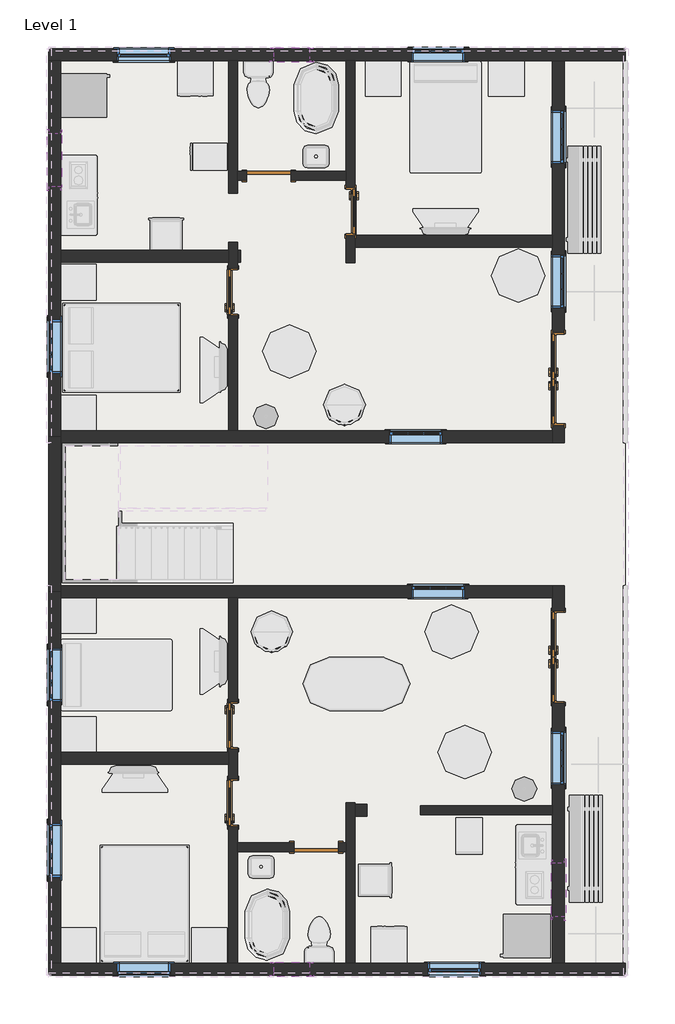
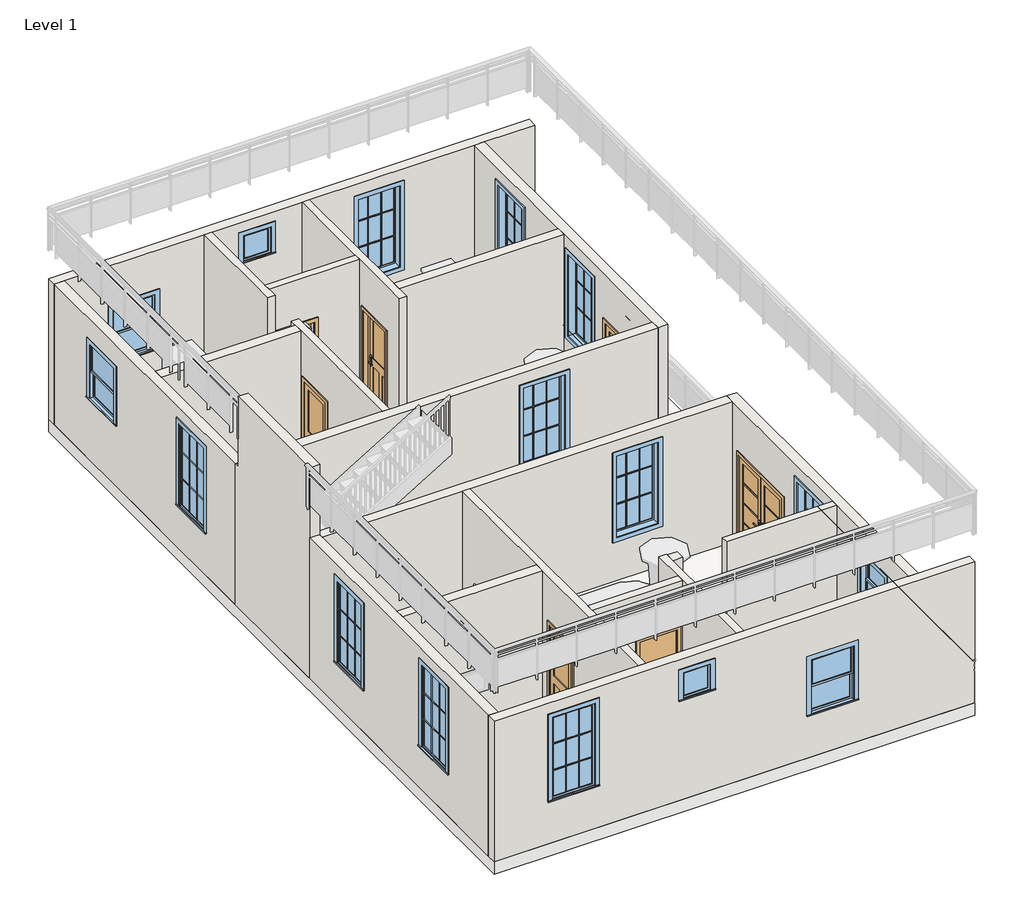
# One storey, part 1 of 4: 22 walls, 16 windows, 8 doors, 1 slab.
"""IFC4 building model written with IfcOpenShell, lengths in millimetres."""

from ifc_helpers import new_model, si_unit, frame, origin, origin_with_axes, place, context, project, spatial, polyline, outline, extrude, faceted_brep, transform, mapped, element, save
from components import door_ce1fc124, door_cdf9d6cc, door_b03bd389, door_255cab33, window_8b323df3, window_31198920, window_e41d21a6

model = new_model("IFC4")

# Units and contexts
model_context = context("Model", 3, world=origin())
ifc_project = project(units=[si_unit("LENGTHUNIT", "METRE", prefix="MILLI")], contexts=[model_context])

# Site, building, storey
site = spatial("IfcSite", under=ifc_project)
building = spatial("IfcBuilding", under=site)
storey = spatial("IfcBuildingStorey", under=building, Name="Level 1", Elevation=0.0)

# Doors
placement = place(None, origin())
door_shape = door_ce1fc124(model_context)
element("IfcDoor", 1, ObjectType="30\" x 80\"", at=placement, inside=storey, context=model_context, shape_type="MappedRepresentation", body=[
    mapped(door_shape, transform((-11423.8500862, 2290.6620171, 0.0), x_axis=(0.0, -1.0, 0.0), y_axis=(1.0, 0.0, 0.0), z_axis=(0.0, 0.0, 1.0))),
])
element("IfcDoor", 2, ObjectType="30\" x 80\"", at=placement, inside=storey, context=model_context, shape_type="MappedRepresentation", body=[
    mapped(door_shape, transform((-11423.8500862, 11015.5620171, 0.0), x_axis=(0.0, -1.0, 0.0), y_axis=(1.0, 0.0, 0.0), z_axis=(0.0, 0.0, 1.0))),
])
element("IfcDoor", 3, ObjectType="30\" x 80\"", at=placement, inside=storey, context=model_context, shape_type="MappedRepresentation", body=[
    mapped(door_shape, transform((-9410.9000862, 12387.1620171, 0.0), x_axis=(0.0, 1.0, 0.0), y_axis=(-1.0, 0.0, 0.0), z_axis=(0.0, 0.0, 1.0))),
])
door_2_shape = door_cdf9d6cc(model_context)
element("IfcDoor", 4, ObjectType="30\" x 80\"", at=placement, inside=storey, context=model_context, shape_type="MappedRepresentation", body=[
    mapped(door_2_shape, transform((-11423.8500862, 3611.4620171, 0.0), x_axis=(0.0, 1.0, 0.0), y_axis=(-1.0, 0.0, 0.0), z_axis=(0.0, 0.0, 1.0))),
])
door_3_shape = door_b03bd389(model_context)
element("IfcDoor", 5, ObjectType="Door-Exterior-Double-Full Glass-Wood_Clad : 60\" x 80\"", at=placement, inside=storey, context=model_context, shape_type="MappedRepresentation", body=[
    mapped(door_3_shape, transform((-5861.2500862, 9529.6620171, 0.0), x_axis=(0.0, 1.0, 0.0), y_axis=(-1.0, 0.0, 0.0), z_axis=(0.0, 0.0, 1.0))),
])
element("IfcDoor", 6, ObjectType="Door-Exterior-Double-Full Glass-Wood_Clad : 60\" x 80\"", at=placement, inside=storey, context=model_context, shape_type="MappedRepresentation", body=[
    mapped(door_3_shape, transform((-5861.2500862, 4779.8620171, 0.0), x_axis=(0.0, 1.0, 0.0), y_axis=(-1.0, 0.0, 0.0), z_axis=(0.0, 0.0, 1.0))),
])
door_4_shape = door_255cab33(model_context)
element("IfcDoor", 7, ObjectType="Single-Flush : 30\" x 80\"", at=placement, inside=storey, context=model_context, shape_type="MappedRepresentation", body=[
    mapped(door_4_shape, transform((-10811.0750862, 12996.7620171, 0.0), x_axis=(-1.0, 0.0, 0.0), y_axis=(0.0, -1.0, 0.0), z_axis=(0.0, 0.0, 1.0))),
])
element("IfcDoor", 8, ObjectType="Single-Flush : 30\" x 80\"", at=placement, inside=storey, context=model_context, shape_type="MappedRepresentation", body=[
    mapped(door_4_shape, transform((-9998.2750862, 1528.6620171, 0.0), x_axis=(1.0, 0.0, 0.0), y_axis=(0.0, 1.0, 0.0), z_axis=(0.0, 0.0, 1.0))),
])

# Slab
element("IfcSlab", 9, ObjectType="Wood Joist 10\" - Ceramic Tile", at=placement, inside=storey, context=model_context, shape_type="SweptSolid", body=[
    extrude(outline(polyline([(-4715.0750862, 15168.4620171), (-4715.0750862, -655.7379829), (-14570.2750862, -655.7379829), (-14570.2750862, 15168.4620171), (-4715.0750862, 15168.4620171)])), frame((0.0, 0.0, -273.05), z_axis=(0.0, 0.0, 1.0), x_axis=(1.0, 0.0, 0.0)), (0.0, 0.0, 1.0), 273.05),
])

# Walls
element("IfcWall", 10, ObjectType="Generic - 8\"", at=placement, inside=storey, context=model_context, shape_type="Brep", body=[
    faceted_brep([(-14570.2750862, 14965.2620171, 0.0), (-14367.0750862, 14965.2620171, 0.0), (-11496.8750862, 14965.2620171, 0.0), (-11344.4750862, 14965.2620171, 0.0), (-9490.2750862, 14965.2620171, 0.0), (-9337.8750862, 14965.2620171, 0.0), (-5959.6750862, 14965.2620171, 0.0), (-5756.4750862, 14965.2620171, 0.0), (-4715.0750862, 14965.2620171, 0.0), (-4715.0750862, 14965.2620171, 3048.0), (-5756.4750862, 14965.2620171, 3048.0), (-5959.6750862, 14965.2620171, 3048.0), (-9337.8750862, 14965.2620171, 3048.0), (-9490.2750862, 14965.2620171, 3048.0), (-11344.4750862, 14965.2620171, 3048.0), (-11496.8750862, 14965.2620171, 3048.0), (-14367.0750862, 14965.2620171, 3048.0), (-14570.2750862, 14965.2620171, 3048.0), (-7458.2750862, 14965.2620171, 2743.2), (-7458.2750862, 14965.2620171, 914.4), (-8372.6750862, 14965.2620171, 914.4), (-8372.6750862, 14965.2620171, 2743.2), (-13401.8750862, 14965.2620171, 2133.6), (-12487.4750862, 14965.2620171, 2133.6), (-12487.4750862, 14965.2620171, 914.4), (-13401.8750862, 14965.2620171, 914.4), (-10722.1750862, 14965.2620171, 2768.6), (-10112.5750862, 14965.2620171, 2768.6), (-10112.5750862, 14965.2620171, 2159.0), (-10722.1750862, 14965.2620171, 2159.0), (-14570.2750862, 15168.4620171, 0.0), (-14570.2750862, 15168.4620171, 3048.0), (-4715.0750862, 15168.4620171, 3048.0), (-4715.0750862, 15168.4620171, 0.0), (-7458.2750862, 15168.4620171, 2743.2), (-8372.6750862, 15168.4620171, 2743.2), (-8372.6750862, 15168.4620171, 914.4), (-7458.2750862, 15168.4620171, 914.4), (-13401.8750862, 15168.4620171, 2133.6), (-13401.8750862, 15168.4620171, 914.4), (-12487.4750862, 15168.4620171, 914.4), (-12487.4750862, 15168.4620171, 2133.6), (-10722.1750862, 15168.4620171, 2768.6), (-10722.1750862, 15168.4620171, 2159.0), (-10112.5750862, 15168.4620171, 2159.0), (-10112.5750862, 15168.4620171, 2768.6)], [[[0, 1, 2, 3, 4, 5, 6, 7, 8, 9, 10, 11, 12, 13, 14, 15, 16, 17], [18, 19, 20, 21], [22, 23, 24, 25], [26, 27, 28, 29]], [[30, 31, 32, 33], [34, 35, 36, 37], [38, 39, 40, 41], [42, 43, 44, 45]], [[8, 7, 6, 5, 4, 3, 2, 1, 0, 30, 33]], [[9, 8, 33, 32]], [[0, 17, 31, 30]], [[19, 18, 34, 37]], [[20, 19, 37, 36]], [[21, 20, 36, 35]], [[18, 21, 35, 34]], [[39, 38, 22, 25]], [[40, 39, 25, 24]], [[41, 40, 24, 23]], [[38, 41, 23, 22]], [[43, 42, 26, 29]], [[44, 43, 29, 28]], [[45, 44, 28, 27]], [[42, 45, 27, 26]], [[17, 16, 15, 14, 13, 12, 11, 10, 9, 32, 31]]]),
])
element("IfcWall", 11, ObjectType="Generic - 8\"", at=placement, inside=storey, context=model_context, shape_type="Brep", body=[
    faceted_brep([(-4715.0750862, -452.5379829, 0.0), (-5756.4750862, -452.5379829, 0.0), (-5959.6750862, -452.5379829, 0.0), (-9337.8750862, -452.5379829, 0.0), (-9490.2750862, -452.5379829, 0.0), (-11344.4750862, -452.5379829, 0.0), (-11496.8750862, -452.5379829, 0.0), (-14367.0750862, -452.5379829, 0.0), (-14570.2750862, -452.5379829, 0.0), (-14570.2750862, -452.5379829, 3048.0), (-14367.0750862, -452.5379829, 3048.0), (-11496.8750862, -452.5379829, 3048.0), (-11344.4750862, -452.5379829, 3048.0), (-9490.2750862, -452.5379829, 3048.0), (-9337.8750862, -452.5379829, 3048.0), (-5959.6750862, -452.5379829, 3048.0), (-5756.4750862, -452.5379829, 3048.0), (-4715.0750862, -452.5379829, 3048.0), (-13401.8750862, -452.5379829, 2743.2), (-13401.8750862, -452.5379829, 914.4), (-12487.4750862, -452.5379829, 914.4), (-12487.4750862, -452.5379829, 2743.2), (-8093.2750862, -452.5379829, 2133.6), (-8093.2750862, -452.5379829, 914.4), (-7178.8750862, -452.5379829, 914.4), (-7178.8750862, -452.5379829, 2133.6), (-10722.1750862, -452.5379829, 2768.6), (-10722.1750862, -452.5379829, 2159.0), (-10112.5750862, -452.5379829, 2159.0), (-10112.5750862, -452.5379829, 2768.6), (-4715.0750862, -655.7379829, 0.0), (-4715.0750862, -655.7379829, 3048.0), (-14570.2750862, -655.7379829, 3048.0), (-14570.2750862, -655.7379829, 0.0), (-13401.8750862, -655.7379829, 2743.2), (-12487.4750862, -655.7379829, 2743.2), (-12487.4750862, -655.7379829, 914.4), (-13401.8750862, -655.7379829, 914.4), (-8093.2750862, -655.7379829, 2133.6), (-7178.8750862, -655.7379829, 2133.6), (-7178.8750862, -655.7379829, 914.4), (-8093.2750862, -655.7379829, 914.4), (-10722.1750862, -655.7379829, 2768.6), (-10112.5750862, -655.7379829, 2768.6), (-10112.5750862, -655.7379829, 2159.0), (-10722.1750862, -655.7379829, 2159.0)], [[[0, 1, 2, 3, 4, 5, 6, 7, 8, 9, 10, 11, 12, 13, 14, 15, 16, 17], [18, 19, 20, 21], [22, 23, 24, 25], [26, 27, 28, 29]], [[30, 31, 32, 33], [34, 35, 36, 37], [38, 39, 40, 41], [42, 43, 44, 45]], [[8, 7, 6, 5, 4, 3, 2, 1, 0, 30, 33]], [[0, 17, 31, 30]], [[9, 8, 33, 32]], [[17, 16, 15, 14, 13, 12, 11, 10, 9, 32, 31]], [[19, 18, 34, 37]], [[20, 19, 37, 36]], [[21, 20, 36, 35]], [[18, 21, 35, 34]], [[23, 22, 38, 41]], [[24, 23, 41, 40]], [[25, 24, 40, 39]], [[22, 25, 39, 38]], [[27, 26, 42, 45]], [[28, 27, 45, 44]], [[29, 28, 44, 43]], [[26, 29, 43, 42]]]),
])
element("IfcWall", 12, ObjectType="Generic - 8\"", at=placement, inside=storey, context=model_context, shape_type="Brep", body=[
    faceted_brep([(-14367.0750862, -452.5379829, 0.0), (-14367.0750862, 2951.0620171, 0.0), (-14367.0750862, 3154.2620171, 0.0), (-14367.0750862, 5795.8620171, 0.0), (-14367.0750862, 5897.4620171, 0.0), (-14367.0750862, 5897.4620171, 3048.0), (-14367.0750862, 5795.8620171, 3048.0), (-14367.0750862, 3154.2620171, 3048.0), (-14367.0750862, 2951.0620171, 3048.0), (-14367.0750862, -452.5379829, 3048.0), (-14367.0750862, 1935.0620171, 2743.2), (-14367.0750862, 1935.0620171, 914.4), (-14367.0750862, 1020.6620171, 914.4), (-14367.0750862, 1020.6620171, 2743.2), (-14367.0750862, 4932.2620171, 2743.2), (-14367.0750862, 4932.2620171, 914.4), (-14367.0750862, 4017.8620171, 914.4), (-14367.0750862, 4017.8620171, 2743.2), (-14570.2750862, -452.5379829, 0.0), (-14570.2750862, -452.5379829, 3048.0), (-14570.2750862, 5897.4620171, 3048.0), (-14570.2750862, 5897.4620171, 0.0), (-14570.2750862, 1935.0620171, 2743.2), (-14570.2750862, 1020.6620171, 2743.2), (-14570.2750862, 1020.6620171, 914.4), (-14570.2750862, 1935.0620171, 914.4), (-14570.2750862, 4932.2620171, 2743.2), (-14570.2750862, 4017.8620171, 2743.2), (-14570.2750862, 4017.8620171, 914.4), (-14570.2750862, 4932.2620171, 914.4)], [[[0, 1, 2, 3, 4, 5, 6, 7, 8, 9], [10, 11, 12, 13], [14, 15, 16, 17]], [[18, 19, 20, 21], [22, 23, 24, 25], [26, 27, 28, 29]], [[4, 3, 2, 1, 0, 18, 21]], [[5, 4, 21, 20]], [[9, 8, 7, 6, 5, 20, 19]], [[0, 9, 19, 18]], [[11, 10, 22, 25]], [[12, 11, 25, 24]], [[13, 12, 24, 23]], [[10, 13, 23, 22]], [[15, 14, 26, 29]], [[16, 15, 29, 28]], [[17, 16, 28, 27]], [[14, 17, 27, 26]]]),
])
element("IfcWall", 13, ObjectType="Generic - 8\"", at=placement, inside=storey, context=model_context, shape_type="Brep", body=[
    faceted_brep([(-5959.6750862, 14965.2620171, 3048.0), (-5959.6750862, 14965.2620171, 0.0), (-5959.6750862, 11980.7620171, 0.0), (-5959.6750862, 11777.5620171, 0.0), (-5959.6750862, 10317.0620171, 0.0), (-5959.6750862, 10317.0620171, 2057.4), (-5959.6750862, 8742.2620171, 2057.4), (-5959.6750862, 8742.2620171, 0.0), (-5959.6750862, 8640.6620171, 0.0), (-5959.6750862, 8437.4620171, 0.0), (-5959.6750862, 8437.4620171, 3048.0), (-5959.6750862, 8640.6620171, 3048.0), (-5959.6750862, 11777.5620171, 3048.0), (-5959.6750862, 11980.7620171, 3048.0), (-5959.6750862, 10736.1620171, 2743.2), (-5959.6750862, 10736.1620171, 914.4), (-5959.6750862, 11650.5620171, 914.4), (-5959.6750862, 11650.5620171, 2743.2), (-5959.6750862, 13206.3120171, 2743.2), (-5959.6750862, 13206.3120171, 914.4), (-5959.6750862, 14120.7120171, 914.4), (-5959.6750862, 14120.7120171, 2743.2), (-5756.4750862, 14965.2620171, 0.0), (-5756.4750862, 14965.2620171, 3048.0), (-5756.4750862, 8437.4620171, 3048.0), (-5756.4750862, 8437.4620171, 0.0), (-5756.4750862, 8742.2620171, 0.0), (-5756.4750862, 8742.2620171, 2057.4), (-5756.4750862, 10317.0620171, 2057.4), (-5756.4750862, 10317.0620171, 0.0), (-5756.4750862, 10736.1620171, 2743.2), (-5756.4750862, 11650.5620171, 2743.2), (-5756.4750862, 11650.5620171, 914.4), (-5756.4750862, 10736.1620171, 914.4), (-5756.4750862, 13206.3120171, 2743.2), (-5756.4750862, 14120.7120171, 2743.2), (-5756.4750862, 14120.7120171, 914.4), (-5756.4750862, 13206.3120171, 914.4)], [[[0, 1, 2, 3, 4, 5, 6, 7, 8, 9, 10, 11, 12, 13], [14, 15, 16, 17], [18, 19, 20, 21]], [[22, 23, 24, 25, 26, 27, 28, 29], [30, 31, 32, 33], [34, 35, 36, 37]], [[1, 22, 29, 4, 3, 2]], [[25, 9, 8, 7, 26]], [[1, 0, 23, 22]], [[10, 9, 25, 24]], [[28, 5, 4, 29]], [[5, 28, 27, 6]], [[6, 27, 26, 7]], [[15, 14, 30, 33]], [[16, 15, 33, 32]], [[17, 16, 32, 31]], [[14, 17, 31, 30]], [[19, 18, 34, 37]], [[20, 19, 37, 36]], [[21, 20, 36, 35]], [[18, 21, 35, 34]], [[0, 13, 12, 11, 10, 24, 23]]]),
])
element("IfcWall", 14, ObjectType="Generic - 8\"", at=placement, inside=storey, context=model_context, shape_type="Brep", body=[
    faceted_brep([(-5959.6750862, 8640.6620171, 0.0), (-11344.4750862, 8640.6620171, 0.0), (-11496.8750862, 8640.6620171, 0.0), (-14367.0750862, 8640.6620171, 0.0), (-14367.0750862, 8640.6620171, 3048.0), (-11496.8750862, 8640.6620171, 3048.0), (-11344.4750862, 8640.6620171, 3048.0), (-5959.6750862, 8640.6620171, 3048.0), (-7839.2750862, 8640.6620171, 2743.2), (-8753.6750862, 8640.6620171, 2743.2), (-8753.6750862, 8640.6620171, 914.4), (-7839.2750862, 8640.6620171, 914.4), (-5959.6750862, 8437.4620171, 0.0), (-5959.6750862, 8437.4620171, 3048.0), (-14367.0750862, 8437.4620171, 3048.0), (-14367.0750862, 8437.4620171, 0.0), (-7839.2750862, 8437.4620171, 2743.2), (-7839.2750862, 8437.4620171, 914.4), (-8753.6750862, 8437.4620171, 914.4), (-8753.6750862, 8437.4620171, 2743.2), (-14367.0750862, 8539.0620171, 0.0), (-14367.0750862, 8539.0620171, 3048.0)], [[[0, 1, 2, 3, 4, 5, 6, 7], [8, 9, 10, 11]], [[12, 13, 14, 15], [16, 17, 18, 19]], [[3, 2, 1, 0, 12, 15, 20]], [[0, 7, 13, 12]], [[17, 16, 8, 11]], [[18, 17, 11, 10]], [[19, 18, 10, 9]], [[16, 19, 9, 8]], [[7, 6, 5, 4, 21, 14, 13]], [[4, 3, 20, 15, 14, 21]]]),
])
element("IfcWall", 15, ObjectType="Generic - 8\"", at=placement, inside=storey, context=model_context, shape_type="Brep", body=[
    faceted_brep([(-5959.6750862, 5999.0620171, 0.0), (-14367.0750862, 5999.0620171, 0.0), (-14367.0750862, 5999.0620171, 3048.0), (-5959.6750862, 5999.0620171, 3048.0), (-7458.2750862, 5999.0620171, 2743.2), (-8372.6750862, 5999.0620171, 2743.2), (-8372.6750862, 5999.0620171, 914.4), (-7458.2750862, 5999.0620171, 914.4), (-5959.6750862, 5795.8620171, 0.0), (-5959.6750862, 5795.8620171, 3048.0), (-11344.4750862, 5795.8620171, 3048.0), (-11496.8750862, 5795.8620171, 3048.0), (-14367.0750862, 5795.8620171, 3048.0), (-14367.0750862, 5795.8620171, 0.0), (-11496.8750862, 5795.8620171, 0.0), (-11344.4750862, 5795.8620171, 0.0), (-7458.2750862, 5795.8620171, 2743.2), (-7458.2750862, 5795.8620171, 914.4), (-8372.6750862, 5795.8620171, 914.4), (-8372.6750862, 5795.8620171, 2743.2), (-14367.0750862, 5897.4620171, 0.0), (-14367.0750862, 5897.4620171, 3048.0)], [[[0, 1, 2, 3], [4, 5, 6, 7]], [[8, 9, 10, 11, 12, 13, 14, 15], [16, 17, 18, 19]], [[1, 0, 8, 15, 14, 13, 20]], [[0, 3, 9, 8]], [[3, 2, 21, 12, 11, 10, 9]], [[17, 16, 4, 7]], [[18, 17, 7, 6]], [[19, 18, 6, 5]], [[16, 19, 5, 4]], [[2, 1, 20, 13, 12, 21]]]),
])
element("IfcWall", 16, ObjectType="Generic - 8\"", at=placement, inside=storey, context=model_context, shape_type="Brep", body=[
    faceted_brep([(-5959.6750862, -452.5379829, 0.0), (-5959.6750862, -452.5379829, 3048.0), (-5959.6750862, 2087.4620171, 3048.0), (-5959.6750862, 2239.8620171, 3048.0), (-5959.6750862, 5795.8620171, 3048.0), (-5959.6750862, 5999.0620171, 3048.0), (-5959.6750862, 5999.0620171, 0.0), (-5959.6750862, 5795.8620171, 0.0), (-5959.6750862, 5567.2620171, 0.0), (-5959.6750862, 5567.2620171, 2057.4), (-5959.6750862, 3992.4620171, 2057.4), (-5959.6750862, 3992.4620171, 0.0), (-5959.6750862, 2239.8620171, 0.0), (-5959.6750862, 2087.4620171, 0.0), (-5959.6750862, 2595.4620171, 2743.2), (-5959.6750862, 2595.4620171, 914.4), (-5959.6750862, 3509.8620171, 914.4), (-5959.6750862, 3509.8620171, 2743.2), (-5959.6750862, 347.5620171, 2540.0), (-5959.6750862, 347.5620171, 1320.8), (-5959.6750862, 1261.9620171, 1320.8), (-5959.6750862, 1261.9620171, 2540.0), (-5756.4750862, -452.5379829, 3048.0), (-5756.4750862, -452.5379829, 0.0), (-5756.4750862, 3992.4620171, 0.0), (-5756.4750862, 3992.4620171, 2057.4), (-5756.4750862, 5567.2620171, 2057.4), (-5756.4750862, 5567.2620171, 0.0), (-5756.4750862, 5999.0620171, 0.0), (-5756.4750862, 5999.0620171, 3048.0), (-5756.4750862, 2595.4620171, 2743.2), (-5756.4750862, 3509.8620171, 2743.2), (-5756.4750862, 3509.8620171, 914.4), (-5756.4750862, 2595.4620171, 914.4), (-5756.4750862, 347.5620171, 2540.0), (-5756.4750862, 1261.9620171, 2540.0), (-5756.4750862, 1261.9620171, 1320.8), (-5756.4750862, 347.5620171, 1320.8)], [[[0, 1, 2, 3, 4, 5, 6, 7, 8, 9, 10, 11, 12, 13], [14, 15, 16, 17], [18, 19, 20, 21]], [[22, 23, 24, 25, 26, 27, 28, 29], [30, 31, 32, 33], [34, 35, 36, 37]], [[23, 0, 13, 12, 11, 24]], [[6, 28, 27, 8, 7]], [[1, 0, 23, 22]], [[6, 5, 29, 28]], [[26, 9, 8, 27]], [[9, 26, 25, 10]], [[10, 25, 24, 11]], [[5, 4, 3, 2, 1, 22, 29]], [[15, 14, 30, 33]], [[16, 15, 33, 32]], [[17, 16, 32, 31]], [[14, 17, 31, 30]], [[19, 18, 34, 37]], [[20, 19, 37, 36]], [[21, 20, 36, 35]], [[18, 21, 35, 34]]]),
])
element("IfcWall", 17, ObjectType="Generic - 8\"", at=placement, inside=storey, context=model_context, shape_type="SweptSolid", body=[
    extrude(outline(polyline([(-14367.0750862, 3154.2620171), (-11496.8750862, 3154.2620171), (-11496.8750862, 2951.0620171), (-14367.0750862, 2951.0620171), (-14367.0750862, 3154.2620171)])), origin_with_axes(), (0.0, 0.0, 1.0), 3048.0),
])
element("IfcWall", 18, ObjectType="Generic - 8\"", at=placement, inside=storey, context=model_context, shape_type="SweptSolid", body=[
    extrude(outline(polyline([(-14367.0750862, 11726.7620171), (-11496.8750862, 11726.7620171), (-11496.8750862, 11523.5620171), (-14367.0750862, 11523.5620171), (-14367.0750862, 11726.7620171)])), origin_with_axes(), (0.0, 0.0, 1.0), 3048.0),
])
element("IfcWall", 19, ObjectType="Generic - 8\"", at=placement, inside=storey, context=model_context, shape_type="SweptSolid", body=[
    extrude(outline(polyline([(-11293.6750862, 11523.5620171), (-11344.4750862, 11523.5620171), (-11344.4750862, 11726.7620171), (-11293.6750862, 11726.7620171), (-11293.6750862, 11523.5620171)])), origin_with_axes(), (0.0, 0.0, 1.0), 3048.0),
])
element("IfcWall", 20, ObjectType="Generic - 8\"", at=placement, inside=storey, context=model_context, shape_type="Brep", body=[
    faceted_brep([(-9337.8750862, 11777.5620171, 0.0), (-5959.6750862, 11777.5620171, 0.0), (-5959.6750862, 11777.5620171, 3048.0), (-9337.8750862, 11777.5620171, 3048.0), (-9337.8750862, 11980.7620171, 0.0), (-9337.8750862, 11980.7620171, 2057.4), (-9337.8750862, 11980.7620171, 3048.0), (-5959.6750862, 11980.7620171, 3048.0), (-5959.6750862, 11980.7620171, 0.0)], [[[0, 1, 2, 3]], [[4, 5, 6, 7, 8]], [[1, 0, 4, 8]], [[2, 1, 8, 7]], [[0, 3, 6, 5, 4]], [[3, 2, 7, 6]]]),
])
element("IfcWall", 21, ObjectType="Generic - 8\"", at=placement, inside=storey, context=model_context, shape_type="SweptSolid", body=[
    extrude(outline(polyline([(-9337.8750862, 2265.2620171), (-9134.6750862, 2265.2620171), (-9134.6750862, 2062.0620171), (-9337.8750862, 2062.0620171), (-9337.8750862, 2265.2620171)])), origin_with_axes(), (0.0, 0.0, 1.0), 3048.0),
])
element("IfcWall", 22, ObjectType="Generic - 8\"", at=placement, inside=storey, context=model_context, shape_type="Brep", body=[
    faceted_brep([(-14367.0750862, 8539.0620171, 0.0), (-14367.0750862, 8640.6620171, 0.0), (-14367.0750862, 11523.5620171, 0.0), (-14367.0750862, 11726.7620171, 0.0), (-14367.0750862, 14965.2620171, 0.0), (-14367.0750862, 14965.2620171, 3048.0), (-14367.0750862, 11726.7620171, 3048.0), (-14367.0750862, 11523.5620171, 3048.0), (-14367.0750862, 8640.6620171, 3048.0), (-14367.0750862, 8539.0620171, 3048.0), (-14367.0750862, 10539.3120171, 2743.2), (-14367.0750862, 10539.3120171, 914.4), (-14367.0750862, 9624.9120171, 914.4), (-14367.0750862, 9624.9120171, 2743.2), (-14367.0750862, 13727.0120171, 2540.0), (-14367.0750862, 13727.0120171, 1320.8), (-14367.0750862, 12812.6120171, 1320.8), (-14367.0750862, 12812.6120171, 2540.0), (-14570.2750862, 8539.0620171, 0.0), (-14570.2750862, 8539.0620171, 3048.0), (-14570.2750862, 14965.2620171, 3048.0), (-14570.2750862, 14965.2620171, 0.0), (-14570.2750862, 10539.3120171, 2743.2), (-14570.2750862, 9624.9120171, 2743.2), (-14570.2750862, 9624.9120171, 914.4), (-14570.2750862, 10539.3120171, 914.4), (-14570.2750862, 13727.0120171, 2540.0), (-14570.2750862, 12812.6120171, 2540.0), (-14570.2750862, 12812.6120171, 1320.8), (-14570.2750862, 13727.0120171, 1320.8)], [[[0, 1, 2, 3, 4, 5, 6, 7, 8, 9], [10, 11, 12, 13], [14, 15, 16, 17]], [[18, 19, 20, 21], [22, 23, 24, 25], [26, 27, 28, 29]], [[4, 3, 2, 1, 0, 18, 21]], [[0, 9, 19, 18]], [[5, 4, 21, 20]], [[10, 13, 23, 22]], [[13, 12, 24, 23]], [[12, 11, 25, 24]], [[11, 10, 22, 25]], [[14, 17, 27, 26]], [[17, 16, 28, 27]], [[16, 15, 29, 28]], [[15, 14, 26, 29]], [[9, 8, 7, 6, 5, 20, 19]]]),
])
element("IfcWall", 23, ObjectType="Generic - 8\"", at=placement, inside=storey, context=model_context, shape_type="Brep", body=[
    faceted_brep([(-14367.0750862, 5897.4620171, 0.0), (-14367.0750862, 5999.0620171, 0.0), (-14367.0750862, 8437.4620171, 0.0), (-14367.0750862, 8539.0620171, 0.0), (-14367.0750862, 8539.0620171, 3048.0), (-14367.0750862, 8437.4620171, 3048.0), (-14367.0750862, 8437.4620171, 4572.0), (-14367.0750862, 5897.4620171, 4572.0), (-14367.0750862, 5897.4620171, 3048.0), (-14570.2750862, 5897.4620171, 0.0), (-14570.2750862, 5897.4620171, 3048.0), (-14570.2750862, 5897.4620171, 4572.0), (-14570.2750862, 8437.4620171, 4572.0), (-14570.2750862, 8437.4620171, 3048.0), (-14570.2750862, 8539.0620171, 3048.0), (-14570.2750862, 8539.0620171, 0.0)], [[[0, 1, 2, 3, 4, 5, 6, 7, 8]], [[9, 10, 11, 12, 13, 14, 15]], [[3, 2, 1, 0, 9, 15]], [[4, 3, 15, 14]], [[0, 8, 7, 11, 10, 9]], [[7, 6, 12, 11]], [[12, 6, 5, 13]], [[5, 4, 14, 13]]]),
])
element("IfcWall", 24, ObjectType="inner wall", at=placement, inside=storey, context=model_context, shape_type="Brep", body=[
    faceted_brep([(-11496.8750862, 14965.2620171, 0.0), (-11496.8750862, 12704.6620171, 0.0), (-11496.8750862, 12704.6620171, 3048.0), (-11496.8750862, 14965.2620171, 3048.0), (-11344.4750862, 14965.2620171, 0.0), (-11344.4750862, 14965.2620171, 3048.0), (-11344.4750862, 13072.9620171, 3048.0), (-11344.4750862, 12920.5620171, 3048.0), (-11344.4750862, 12704.6620171, 3048.0), (-11344.4750862, 12704.6620171, 0.0), (-11344.4750862, 12920.5620171, 0.0), (-11344.4750862, 13072.9620171, 0.0)], [[[0, 1, 2, 3]], [[4, 5, 6, 7, 8, 9, 10, 11]], [[1, 0, 4, 11, 10, 9]], [[2, 1, 9, 8]], [[0, 3, 5, 4]], [[3, 2, 8, 7, 6, 5]]]),
])
element("IfcWall", 25, ObjectType="inner wall", at=placement, inside=storey, context=model_context, shape_type="Brep", body=[
    faceted_brep([(-9490.2750862, 11510.8620171, 0.0), (-9490.2750862, 11510.8620171, 3048.0), (-9490.2750862, 12920.5620171, 3048.0), (-9490.2750862, 13072.9620171, 3048.0), (-9490.2750862, 14965.2620171, 3048.0), (-9490.2750862, 14965.2620171, 0.0), (-9490.2750862, 13072.9620171, 0.0), (-9490.2750862, 12920.5620171, 0.0), (-9490.2750862, 12793.5620171, 0.0), (-9490.2750862, 12793.5620171, 2057.4), (-9490.2750862, 11980.7620171, 2057.4), (-9490.2750862, 11980.7620171, 0.0), (-9337.8750862, 11510.8620171, 3048.0), (-9337.8750862, 11510.8620171, 0.0), (-9337.8750862, 11777.5620171, 0.0), (-9337.8750862, 11980.7620171, 0.0), (-9337.8750862, 11980.7620171, 2057.4), (-9337.8750862, 12793.5620171, 2057.4), (-9337.8750862, 12793.5620171, 0.0), (-9337.8750862, 14965.2620171, 0.0), (-9337.8750862, 14965.2620171, 3048.0), (-9337.8750862, 11980.7620171, 3048.0), (-9337.8750862, 11777.5620171, 3048.0)], [[[0, 1, 2, 3, 4, 5, 6, 7, 8, 9, 10, 11]], [[12, 13, 14, 15, 16, 17, 18, 19, 20, 21, 22]], [[13, 0, 11, 15, 14]], [[5, 19, 18, 8, 7, 6]], [[1, 0, 13, 12]], [[5, 4, 20, 19]], [[17, 9, 8, 18]], [[9, 17, 16, 10]], [[10, 16, 15, 11]], [[4, 3, 2, 1, 12, 22, 21, 20]]]),
])
element("IfcWall", 26, ObjectType="inner wall", at=placement, inside=storey, context=model_context, shape_type="Brep", body=[
    faceted_brep([(-11496.8750862, -452.5379829, 0.0), (-11496.8750862, -452.5379829, 3048.0), (-11496.8750862, 2951.0620171, 3048.0), (-11496.8750862, 3154.2620171, 3048.0), (-11496.8750862, 5795.8620171, 3048.0), (-11496.8750862, 5795.8620171, 0.0), (-11496.8750862, 4017.8620171, 0.0), (-11496.8750862, 4017.8620171, 2057.4), (-11496.8750862, 3205.0620171, 2057.4), (-11496.8750862, 3205.0620171, 0.0), (-11496.8750862, 3154.2620171, 0.0), (-11496.8750862, 2951.0620171, 0.0), (-11496.8750862, 2697.0620171, 0.0), (-11496.8750862, 2697.0620171, 2057.4), (-11496.8750862, 1884.2620171, 2057.4), (-11496.8750862, 1884.2620171, 0.0), (-11344.4750862, -452.5379829, 3048.0), (-11344.4750862, -452.5379829, 0.0), (-11344.4750862, 1452.4620171, 0.0), (-11344.4750862, 1604.8620171, 0.0), (-11344.4750862, 1884.2620171, 0.0), (-11344.4750862, 1884.2620171, 2057.4), (-11344.4750862, 2697.0620171, 2057.4), (-11344.4750862, 2697.0620171, 0.0), (-11344.4750862, 3205.0620171, 0.0), (-11344.4750862, 3205.0620171, 2057.4), (-11344.4750862, 4017.8620171, 2057.4), (-11344.4750862, 4017.8620171, 0.0), (-11344.4750862, 5795.8620171, 0.0), (-11344.4750862, 5795.8620171, 3048.0), (-11344.4750862, 1604.8620171, 3048.0), (-11344.4750862, 1452.4620171, 3048.0)], [[[0, 1, 2, 3, 4, 5, 6, 7, 8, 9, 10, 11, 12, 13, 14, 15]], [[16, 17, 18, 19, 20, 21, 22, 23, 24, 25, 26, 27, 28, 29, 30, 31]], [[17, 0, 15, 20, 19, 18]], [[5, 28, 27, 6]], [[23, 12, 11, 10, 9, 24]], [[1, 0, 17, 16]], [[5, 4, 29, 28]], [[14, 21, 20, 15]], [[21, 14, 13, 22]], [[22, 13, 12, 23]], [[26, 7, 6, 27]], [[7, 26, 25, 8]], [[8, 25, 24, 9]], [[4, 3, 2, 1, 16, 31, 30, 29]]]),
])
element("IfcWall", 27, ObjectType="inner wall", at=placement, inside=storey, context=model_context, shape_type="SweptSolid", body=[
    extrude(outline(polyline([(0.0, -11344.4750862), (0.0, -11192.0750862), (2032.0, -11192.0750862), (2032.0, -10430.0750862), (0.0, -10430.0750862), (0.0, -9490.2750862), (3048.0, -9490.2750862), (3048.0, -11344.4750862), (0.0, -11344.4750862)])), frame((0.0, 12920.5620171, 0.0), z_axis=(0.0, 1.0, 0.0), x_axis=(0.0, 0.0, 1.0)), (0.0, 0.0, 1.0), 152.4),
])
element("IfcWall", 28, ObjectType="inner wall", at=placement, inside=storey, context=model_context, shape_type="SweptSolid", body=[
    extrude(outline(polyline([(-8220.2750862, 2239.8620171), (-5959.6750862, 2239.8620171), (-5959.6750862, 2087.4620171), (-8220.2750862, 2087.4620171), (-8220.2750862, 2239.8620171)])), origin_with_axes(), (0.0, 0.0, 1.0), 3048.0),
])
element("IfcWall", 29, ObjectType="inner wall", at=placement, inside=storey, context=model_context, shape_type="SweptSolid", body=[
    extrude(outline(polyline([(2032.0, -9617.2750862), (0.0, -9617.2750862), (0.0, -9490.2750862), (3048.0, -9490.2750862), (3048.0, -11344.4750862), (0.0, -11344.4750862), (0.0, -10379.2750862), (2032.0, -10379.2750862), (2032.0, -9617.2750862)])), frame((0.0, 1452.4620171, 0.0), z_axis=(0.0, 1.0, 0.0), x_axis=(0.0, 0.0, 1.0)), (0.0, 0.0, 1.0), 152.4),
])
element("IfcWall", 30, ObjectType="inner wall", at=placement, inside=storey, context=model_context, shape_type="Brep", body=[
    faceted_brep([(-11496.8750862, 11866.4620171, 3048.0), (-11496.8750862, 11866.4620171, 0.0), (-11496.8750862, 11726.7620171, 0.0), (-11496.8750862, 11523.5620171, 0.0), (-11496.8750862, 11421.9620171, 0.0), (-11496.8750862, 11421.9620171, 2057.4), (-11496.8750862, 10609.1620171, 2057.4), (-11496.8750862, 10609.1620171, 0.0), (-11496.8750862, 8640.6620171, 0.0), (-11496.8750862, 8640.6620171, 3048.0), (-11496.8750862, 11523.5620171, 3048.0), (-11496.8750862, 11726.7620171, 3048.0), (-11344.4750862, 11866.4620171, 0.0), (-11344.4750862, 11866.4620171, 3048.0), (-11344.4750862, 11726.7620171, 3048.0), (-11344.4750862, 11523.5620171, 3048.0), (-11344.4750862, 8640.6620171, 3048.0), (-11344.4750862, 8640.6620171, 0.0), (-11344.4750862, 10609.1620171, 0.0), (-11344.4750862, 10609.1620171, 2057.4), (-11344.4750862, 11421.9620171, 2057.4), (-11344.4750862, 11421.9620171, 0.0), (-11344.4750862, 11523.5620171, 0.0), (-11344.4750862, 11726.7620171, 0.0)], [[[0, 1, 2, 3, 4, 5, 6, 7, 8, 9, 10, 11]], [[12, 13, 14, 15, 16, 17, 18, 19, 20, 21, 22, 23]], [[1, 12, 23, 22, 21, 4, 3, 2]], [[17, 8, 7, 18]], [[1, 0, 13, 12]], [[9, 8, 17, 16]], [[6, 19, 18, 7]], [[19, 6, 5, 20]], [[20, 5, 4, 21]], [[0, 11, 10, 9, 16, 15, 14, 13]]]),
])
element("IfcWall", 31, ObjectType="inner wall", at=placement, inside=storey, context=model_context, shape_type="Brep", body=[
    faceted_brep([(-9490.2750862, 2290.6620171, 0.0), (-9490.2750862, 1604.8620171, 0.0), (-9490.2750862, 1452.4620171, 0.0), (-9490.2750862, -452.5379829, 0.0), (-9490.2750862, -452.5379829, 3048.0), (-9490.2750862, 1452.4620171, 3048.0), (-9490.2750862, 1604.8620171, 3048.0), (-9490.2750862, 2290.6620171, 3048.0), (-9337.8750862, 2290.6620171, 0.0), (-9337.8750862, 2290.6620171, 3048.0), (-9337.8750862, 2265.2620171, 3048.0), (-9337.8750862, 2062.0620171, 3048.0), (-9337.8750862, -452.5379829, 3048.0), (-9337.8750862, -452.5379829, 0.0), (-9337.8750862, 2062.0620171, 0.0), (-9337.8750862, 2265.2620171, 0.0)], [[[0, 1, 2, 3, 4, 5, 6, 7]], [[8, 9, 10, 11, 12, 13, 14, 15]], [[3, 2, 1, 0, 8, 15, 14, 13]], [[0, 7, 9, 8]], [[4, 3, 13, 12]], [[7, 6, 5, 4, 12, 11, 10, 9]]]),
])

# Windows
window_shape = window_8b323df3(model_context)
element("IfcWindow", 32, ObjectType="Casement 3x3 with Trim : 36\" x 72\"", at=placement, inside=storey, context=model_context, shape_type="MappedRepresentation", body=[
    mapped(window_shape, transform((-14468.6750862, 1477.8620171, 609.6), x_axis=(0.0, 1.0, 0.0), y_axis=(-1.0, 0.0, 0.0), z_axis=(0.0, 0.0, 1.0))),
])
element("IfcWindow", 33, ObjectType="Casement 3x3 with Trim : 36\" x 72\"", at=placement, inside=storey, context=model_context, shape_type="MappedRepresentation", body=[
    mapped(window_shape, transform((-12944.6750862, -554.1379829, 609.6), x_axis=(-1.0, 0.0, 0.0), y_axis=(0.0, -1.0, 0.0), z_axis=(0.0, 0.0, 1.0))),
])
element("IfcWindow", 34, ObjectType="Casement 3x3 with Trim : 36\" x 72\"", at=placement, inside=storey, context=model_context, shape_type="MappedRepresentation", body=[
    mapped(window_shape, transform((-14468.6750862, 4475.0620171, 609.6), x_axis=(0.0, 1.0, 0.0), y_axis=(-1.0, 0.0, 0.0), z_axis=(0.0, 0.0, 1.0))),
])
element("IfcWindow", 35, ObjectType="Casement 3x3 with Trim : 36\" x 72\"", at=placement, inside=storey, context=model_context, shape_type="MappedRepresentation", body=[
    mapped(window_shape, transform((-5858.0750862, 3052.6620171, 609.6), x_axis=(0.0, -1.0, 0.0), y_axis=(1.0, 0.0, 0.0), z_axis=(0.0, 0.0, 1.0))),
])
element("IfcWindow", 36, ObjectType="Casement 3x3 with Trim : 36\" x 72\"", at=placement, inside=storey, context=model_context, shape_type="MappedRepresentation", body=[
    mapped(window_shape, transform((-7915.4750862, 5897.4620171, 609.6), x_axis=(1.0, 0.0, 0.0), y_axis=(0.0, 1.0, 0.0), z_axis=(0.0, 0.0, 1.0))),
])
element("IfcWindow", 37, ObjectType="Casement 3x3 with Trim : 36\" x 72\"", at=placement, inside=storey, context=model_context, shape_type="MappedRepresentation", body=[
    mapped(window_shape, transform((-8296.4750862, 8539.0620171, 609.6), x_axis=(1.0, 0.0, 0.0), y_axis=(0.0, 1.0, 0.0), z_axis=(0.0, 0.0, 1.0))),
])
element("IfcWindow", 38, ObjectType="Casement 3x3 with Trim : 36\" x 72\"", at=placement, inside=storey, context=model_context, shape_type="MappedRepresentation", body=[
    mapped(window_shape, transform((-5858.0750862, 11193.3620171, 609.6), x_axis=(0.0, -1.0, 0.0), y_axis=(1.0, 0.0, 0.0), z_axis=(0.0, 0.0, 1.0))),
])
element("IfcWindow", 39, ObjectType="Casement 3x3 with Trim : 36\" x 72\"", at=placement, inside=storey, context=model_context, shape_type="MappedRepresentation", body=[
    mapped(window_shape, transform((-5858.0750862, 13663.5120171, 609.6), x_axis=(0.0, -1.0, 0.0), y_axis=(1.0, 0.0, 0.0), z_axis=(0.0, 0.0, 1.0))),
])
element("IfcWindow", 40, ObjectType="Casement 3x3 with Trim : 36\" x 72\"", at=placement, inside=storey, context=model_context, shape_type="MappedRepresentation", body=[
    mapped(window_shape, transform((-7915.4750862, 15066.8620171, 609.6), x_axis=(1.0, 0.0, 0.0), y_axis=(0.0, 1.0, 0.0), z_axis=(0.0, 0.0, 1.0))),
])
element("IfcWindow", 41, ObjectType="Casement 3x3 with Trim : 36\" x 72\"", at=placement, inside=storey, context=model_context, shape_type="MappedRepresentation", body=[
    mapped(window_shape, transform((-14468.6750862, 10082.1120171, 609.6), x_axis=(0.0, 1.0, 0.0), y_axis=(-1.0, 0.0, 0.0), z_axis=(0.0, 0.0, 1.0))),
])
window_2_shape = window_31198920(model_context)
element("IfcWindow", 42, ObjectType="Double Hung with Trim : 36\" x 48\"", at=placement, inside=storey, context=model_context, shape_type="MappedRepresentation", body=[
    mapped(window_2_shape, transform((-5858.0750862, 804.7620171, 406.4), x_axis=(0.0, -1.0, 0.0), y_axis=(1.0, 0.0, 0.0), z_axis=(0.0, 0.0, 1.0))),
])
element("IfcWindow", 43, ObjectType="Double Hung with Trim : 36\" x 48\"", at=placement, inside=storey, context=model_context, shape_type="MappedRepresentation", body=[
    mapped(window_2_shape, transform((-7636.0750862, -554.1379829, 0.0), x_axis=(-1.0, 0.0, 0.0), y_axis=(0.0, -1.0, 0.0), z_axis=(0.0, 0.0, 1.0))),
])
element("IfcWindow", 44, ObjectType="Double Hung with Trim : 36\" x 48\"", at=placement, inside=storey, context=model_context, shape_type="MappedRepresentation", body=[
    mapped(window_2_shape, transform((-12944.6750862, 15066.8620171, 0.0), x_axis=(-1.0, 0.0, 0.0), y_axis=(0.0, -1.0, 0.0), z_axis=(0.0, 0.0, 1.0))),
])
element("IfcWindow", 45, ObjectType="Double Hung with Trim : 36\" x 48\"", at=placement, inside=storey, context=model_context, shape_type="MappedRepresentation", body=[
    mapped(window_2_shape, transform((-14468.6750862, 13269.8120171, 406.4), x_axis=(0.0, 1.0, 0.0), y_axis=(-1.0, 0.0, 0.0), z_axis=(0.0, 0.0, 1.0))),
])
window_3_shape = window_e41d21a6(model_context)
element("IfcWindow", 46, ObjectType="Transom with Trim : 24\" x 24\"", at=placement, inside=storey, context=model_context, shape_type="MappedRepresentation", body=[
    mapped(window_3_shape, transform((-10455.4750862, -554.1379829, 0.0), x_axis=(-1.0, 0.0, 0.0), y_axis=(0.0, -1.0, 0.0), z_axis=(0.0, 0.0, 1.0))),
])
element("IfcWindow", 47, ObjectType="Transom with Trim : 24\" x 24\"", at=placement, inside=storey, context=model_context, shape_type="MappedRepresentation", body=[
    mapped(window_3_shape, transform((-10455.4750862, 15066.8620171, 0.0), x_axis=(-1.0, 0.0, 0.0), y_axis=(0.0, -1.0, 0.0), z_axis=(0.0, 0.0, 1.0))),
])

save(model, "model.ifc")

# Revit data of these elements
# Type "30\" x 80\""
#   Type Mark = "9"
#   Assembly Code = "B2030100"
#   Analytic Construction = "French door, wood frame with single glass"
#   Top Rail = 0' - 4 3/4"
#   Threshold Offset [instance default] = 0' - 0 1/2"
#   Thickness = 0' - 1 3/8"
#   Thermal Resistance (R) = 1.0696 (h·ft²·°F)/BTU
#   Swing Angle [instance default] = 90.00°
#   Stiles = 0' - 4 3/4"
#   Rough Width = 2' - 8"
#   Rough Height = 6' - 9"
#   Lock Rail = 0' - 7 1/8"
#   Height = 6' - 8"
#   Width = 2' - 6"
#   Heat Transfer Coefficient (U) = 0.9350 BTU/(h·ft²·°F)
#   Door Offset [instance default] = 0' - 0"
#   Bottom Rail = 0' - 9 1/2"
#   Threshold [instance default] = yes
#   Function = 1
#   Exterior Trim [instance default] = yes
#   Trim Material = Cherry
#   Threshold Material = Cherry
#   Panel Material = Cherry
#   Glazing = Glass
#   Frame Material = Cherry
#   Door Handle Material = Aluminum
#   Visual Light Transmittance = 0
#   Solar Heat Gain Coefficient = 0
#   Wall Closure = (empty or 0)
#   Construction Type = (empty or 0)
# Type "Door-Exterior-Double-Full Glass-Wood_Clad : 60\" x 80\""
#   Type Mark = "8"
#   Assembly Code = "B2030100"
#   Analytic Construction = "French door, wood frame with double glass"
#   Top Rail = 0' - 4 11/16"
#   Threshold Offset [instance default] = 0' - 0 1/2"
#   Thickness = 0' - 1 3/8"
#   Thermal Resistance (R) = 1.9158 (h·ft²·°F)/BTU
#   Swing Angle [instance default] = 90.00°
#   Stiles = 0' - 4 3/4"
#   Rough Width = 5' - 2"
#   Rough Height = 6' - 9"
#   Panel Width = 2' - 6"
#   Door Offset [instance default] = 0' - 0"
#   Height = 6' - 8"
#   Width = 5' - 0"
#   Heat Transfer Coefficient (U) = 0.5220 BTU/(h·ft²·°F)
#   Bottom Rail = 0' - 9 1/8"
#   Exterior Trim [instance default] = yes
#   Threshold [instance default] = yes
#   Show Grill [instance default] = yes
#   Function = 1
#   Trim Material = Cherry
#   Threshold Material = Cherry
#   Panel Material = Cherry
#   Glazing = Glass
#   Frame Material = Cherry
#   Door Handle Material = Aluminum
#   Visual Light Transmittance = 0
#   Solar Heat Gain Coefficient = 0
#   Wall Closure = (empty or 0)
#   Construction Type = (empty or 0)
# Type "Single-Flush : 30\" x 80\""
#   Type Mark = "5"
#   Construction Type Id = "MDOOR"
#   Assembly Code = "C1020"
#   Analytic Construction = "Metal"
#   Thickness = 0' - 2"
#   Heat Transfer Coefficient (U) = 0.651978 BTU/(h·ft²·°F)
#   Height = 6' - 8"
#   Trim Projection Ext = 0' - 1"
#   Trim Projection Int = 0' - 1"
#   Trim Width = 0' - 3"
#   Width = 2' - 6"
#   Define Thermal Properties by = 1
#   Door Material = Door - Panel
#   Frame Material = Door - Frame
#   Visual Light Transmittance = 0
#   Solar Heat Gain Coefficient = 0
#   Function = (empty or 0)
#   Wall Closure = (empty or 0)
# Type "Wood Joist 10\" - Ceramic Tile"
#   Assembly Code = "B1010"
#   Function = 0
#   Layers, outside or top first: 0' - 0 1/4" "Tile, Mosaic, Gray" (function 5); 0' - 0 1/2" "Concrete, Cast-in-Place gray" (function 4); 0' - 0 3/4" "Plywood, Sheathing" (function 1); 0' - 9 1/4" "Structure, Wood Joist/Rafter Layer" (function 1)
# Type "Generic - 8\""
#   Assembly Code = "B2010"
#   Layers, outside or top first: 0' - 8" "Birch" (function 1)
# Type "inner wall"
#   Assembly Code = "B2010"
#   Layers, outside or top first: 0' - 6" "Birch" (function 1)
# Type "Casement 3x3 with Trim : 36\" x 72\""
#   Type Mark = "12"
#   Construction Type Id = "GSP4R"
#   Assembly Code = "B2020100"
#   Analytic Construction = "1/8 in Pilkington single glazing"
#   Visual Light Transmittance = 0.9
#   Solar Heat Gain Coefficient = 0.78
#   Heat Transfer Coefficient (U) = 0.6496 BTU/(h·ft²·°F)
#   Height = 6' - 0"
#   Default Sill Height = 1' - 0"
#   Trim Projection - Ext. = 0' - 0 1/2"
#   Trim Projection - Int. = 0' - 0 3/4"
#   Trim Width - Exterior = 0' - 3 1/2"
#   Trim Width - Interior = 0' - 3 1/2"
#   Width = 3' - 0"
#   Window Inset = 0' - 0 3/4"
#   Define Thermal Properties by = 1
#   Glass Pane Material = Glass
#   Sash Material = Sash
#   Trim Exterior Material = Trim
#   Trim Interior Material = Trim
#   Wall Closure = (empty or 0)
# Type "Double Hung with Trim : 36\" x 48\""
#   Type Mark = "13"
#   Construction Type Id = "GSP4R"
#   Assembly Code = "B2020100"
#   Analytic Construction = "1/8 in Pilkington single glazing"
#   Visual Light Transmittance = 0.9
#   Solar Heat Gain Coefficient = 0.78
#   Heat Transfer Coefficient (U) = 0.6496 BTU/(h·ft²·°F)
#   Height = 4' - 0"
#   Default Sill Height = 3' - 0"
#   Trim Projection - Ext. = 0' - 0 1/2"
#   Trim Projection - Int. = 0' - 0 3/4"
#   Trim Width - Exterior = 0' - 3 1/2"
#   Trim Width - Interior = 0' - 3 1/2"
#   Width = 3' - 0"
#   Window Inset = 0' - 0 3/4"
#   Define Thermal Properties by = 1
#   Glass Pane Material = Glass
#   Sash Material = Sash
#   Trim Exterior Material = Trim
#   Trim Interior Material = Trim
#   Wall Closure = (empty or 0)
# Type "Transom with Trim : 24\" x 24\""
#   Type Mark = "22"
#   Construction Type Id = "GSP4R"
#   Assembly Code = "B2020100"
#   Analytic Construction = "1/8 in Pilkington single glazing"
#   Visual Light Transmittance = 0.9
#   Solar Heat Gain Coefficient = 0.78
#   Heat Transfer Coefficient (U) = 0.6496 BTU/(h·ft²·°F)
#   Height = 2' - 0"
#   Default Sill Height = 7' - 1"
#   Trim Projection - Ext. = 0' - 0 1/2"
#   Trim Projection - Int. = 0' - 0 3/4"
#   Trim Width - Exterior = 0' - 3 1/2"
#   Trim Width - Interior = 0' - 3 1/2"
#   Width = 2' - 0"
#   Window Inset = 0' - 0 3/4"
#   Define Thermal Properties by = 1
#   Glass Pane Material = Glass
#   Sash Material = Sash
#   Trim Exterior Material = Trim
#   Trim Interior Material = Trim
#   Wall Closure = (empty or 0)
# Elements 1, 2, 3, 4 (IfcDoor, "30\" x 80\"")
#   Threshold Offset = 0' - 0 1/2"
#   Swing Angle = 90.00°
#   Door Offset = 0' - 0"
#   Threshold = yes
#   Exterior Trim = yes
#   Phase Created = New Construction
#   Materials on its faces: "Cherry", "Aluminum", "Glass"
# Elements 5, 6 (IfcDoor, "Door-Exterior-Double-Full Glass-Wood_Clad : 60\" x 80\"")
#   Threshold Offset = 0' - 0 1/2"
#   Swing Angle = 90.00°
#   Door Offset = 0' - 0"
#   Threshold = yes
#   Show Grill = yes
#   Exterior Trim = yes
#   Phase Created = New Construction
#   Materials on its faces: "Cherry", "Aluminum", "Glass"
# Elements 7, 8 (IfcDoor, "Single-Flush : 30\" x 80\"")
#   Phase Created = New Construction
#   Materials on its faces: "Door - Frame", "Door - Panel"
# Element 9 (IfcSlab, "Wood Joist 10\" - Ceramic Tile")
#   Height Offset From Level = 0' - 0"
#   Phase Created = New Construction
#   Materials on its faces: "Structure, Wood Joist/Rafter Layer", "Tile, Mosaic, Gray"
# Elements 10, 11, 12, 13, 14, 15, 16, 17, 18, 19, 20, 21, 22 (IfcWall, "Generic - 8\"")
#   Top Offset = 0' - 0"
#   Base Offset = 0' - 0"
#   Unconnected Height = 10' - 0"
#   wall height = 10' - 0"
#   Phase Created = New Construction
#   Base Constraint = Level 1
#   Materials on its faces: "Birch"
# Element 23 (IfcWall, "Generic - 8\"")
#   Top Offset = 0' - 0"
#   Base Offset = 0' - 0"
#   Unconnected Height = 15' - 0"
#   wall height = 15' - 0"
#   Phase Created = New Construction
#   Base Constraint = Level 1
#   Materials on its faces: "Birch"
# Elements 24, 25, 26, 27, 28, 29, 30, 31 (IfcWall, "inner wall")
#   Top Offset = 0' - 0"
#   Base Offset = 0' - 0"
#   Unconnected Height = 10' - 0"
#   wall height = 10' - 0"
#   Phase Created = New Construction
#   Base Constraint = Level 1
#   Materials on its faces: "Birch"
# Element 32 (IfcWindow, "Casement 3x3 with Trim : 36\" x 72\"")
#   Mark = "1"
#   Phase Created = New Construction
#   Materials on its faces: "Sash", "Glass", "Trim"
# Element 33 (IfcWindow, "Casement 3x3 with Trim : 36\" x 72\"")
#   Mark = "2"
#   Phase Created = New Construction
#   Materials on its faces: "Sash", "Glass", "Trim"
# Element 34 (IfcWindow, "Casement 3x3 with Trim : 36\" x 72\"")
#   Mark = "3"
#   Phase Created = New Construction
#   Materials on its faces: "Sash", "Glass", "Trim"
# Element 35 (IfcWindow, "Casement 3x3 with Trim : 36\" x 72\"")
#   Mark = "4"
#   Phase Created = New Construction
#   Materials on its faces: "Sash", "Glass", "Trim"
# Element 36 (IfcWindow, "Casement 3x3 with Trim : 36\" x 72\"")
#   Mark = "5"
#   Phase Created = New Construction
#   Materials on its faces: "Sash", "Glass", "Trim"
# Element 37 (IfcWindow, "Casement 3x3 with Trim : 36\" x 72\"")
#   Mark = "6"
#   Phase Created = New Construction
#   Materials on its faces: "Sash", "Glass", "Trim"
# Element 38 (IfcWindow, "Casement 3x3 with Trim : 36\" x 72\"")
#   Mark = "7"
#   Phase Created = New Construction
#   Materials on its faces: "Sash", "Glass", "Trim"
# Element 39 (IfcWindow, "Casement 3x3 with Trim : 36\" x 72\"")
#   Mark = "8"
#   Phase Created = New Construction
#   Materials on its faces: "Sash", "Glass", "Trim"
# Element 40 (IfcWindow, "Casement 3x3 with Trim : 36\" x 72\"")
#   Mark = "9"
#   Phase Created = New Construction
#   Materials on its faces: "Sash", "Glass", "Trim"
# Element 41 (IfcWindow, "Casement 3x3 with Trim : 36\" x 72\"")
#   Mark = "12"
#   Phase Created = New Construction
#   Materials on its faces: "Sash", "Glass", "Trim"
# Element 42 (IfcWindow, "Double Hung with Trim : 36\" x 48\"")
#   Mark = "13"
#   Phase Created = New Construction
#   Materials on its faces: "Sash", "Trim", "Glass"
# Element 43 (IfcWindow, "Double Hung with Trim : 36\" x 48\"")
#   Mark = "14"
#   Phase Created = New Construction
#   Materials on its faces: "Sash", "Trim", "Glass"
# Element 44 (IfcWindow, "Double Hung with Trim : 36\" x 48\"")
#   Mark = "15"
#   Phase Created = New Construction
#   Materials on its faces: "Sash", "Trim", "Glass"
# Element 45 (IfcWindow, "Double Hung with Trim : 36\" x 48\"")
#   Mark = "16"
#   Phase Created = New Construction
#   Materials on its faces: "Sash", "Trim", "Glass"
# Element 46 (IfcWindow, "Transom with Trim : 24\" x 24\"")
#   Mark = "17"
#   Phase Created = New Construction
#   Materials on its faces: "Sash", "Trim", "Glass"
# Element 47 (IfcWindow, "Transom with Trim : 24\" x 24\"")
#   Mark = "18"
#   Phase Created = New Construction
#   Materials on its faces: "Sash", "Trim", "Glass"
# Materials
#   "Cherry": class "Wood", colour RGB 226 177 128, transparency 0, Description = "Prunus Serotina", Cost = 0
#   "Glass": class "Glass", colour RGB 0 128 192, transparency 0.75, Description = "Soda Lime Glass", Cost = 0
#   "Aluminum": class "Metal", colour RGB 247 247 247, transparency 0, Description = "Aluminum 6061", Cost = 0
#   "Door - Panel": class "Wood", colour RGB 210 159 95, transparency 0
#   "Door - Frame": colour RGB 118 70 51, transparency 0
#   "Tile, Mosaic, Gray": class "Generic", colour RGB 127 127 127, transparency 0, Description = "Mosiac tile, gray", Cost = 0
#   "Concrete, Cast-in-Place gray": class "Concrete", colour RGB 192 192 192, transparency 0, Description = "Cast-in-place concrete", Cost = 0
#   "Plywood, Sheathing": class "Wood", colour RGB 212 179 113, transparency 0, Description = "Plywood, sheathing grade", Cost = 0
#   "Structure, Wood Joist/Rafter Layer": class "Wood", colour RGB 127 127 127, transparency 0, Description = "Wood framing, thermal airspace", Cost = 0
#   "Birch": class "Wood", colour RGB 224 178 126, transparency 0, Description = "Betula Alleghaniensis", Cost = 0
#   "Sash": class "Wood", colour RGB 224 178 126, transparency 0
#   "Trim": class "Wood", colour RGB 224 178 126, transparency 0
# Room at (-5090.973, 2809.393) mm, phase "New Construction", upper level "Level 1", upper offset 10' - 0", lower offset 0' - 0"
#   Number = "1"
#   Name = "WIDE PASSAGE"
# Room at (-5066.841, 11528.389) mm, phase "New Construction", upper level "Level 1", upper offset 10' - 0", lower offset 0' - 0"
#   Number = "2"
#   Name = "WIDE PASSAGE"
# Room at (-8872.341, 7107.17) mm, phase "New Construction", upper level "Level 1", upper offset 10' - 0", lower offset 0' - 0"
#   Number = "3"
#   Name = "WIDE PASSAGE"
# Room at (-8872.341, 4103.824) mm, phase "New Construction", upper level "Level 1", upper offset 10' - 0", lower offset 0' - 0"
#   Number = "4"
#   Name = "LIVING HALL"
# Room at (-7648.246, 816.724) mm, phase "New Construction", upper level "Level 1", upper offset 10' - 0", lower offset 0' - 0"
#   Number = "5"
#   Name = "KITCHEN"
# Room at (-13128.804, 1424.533) mm, phase "New Construction", upper level "Level 1", upper offset 10' - 0", lower offset 0' - 0"
#   Number = "6"
#   Name = "M BED ROOM"
# Room at (-13128.804, 4745.432) mm, phase "New Construction", upper level "Level 1", upper offset 10' - 0", lower offset 0' - 0"
#   Number = "7"
#   Name = "BED ROOM 1"
# Room at (-10318.813, 530.445) mm, phase "New Construction", upper level "Level 1", upper offset 10' - 0", lower offset 0' - 0"
#   Number = "8"
#   Name = "TOILET"
# Room at (-13128.804, 10115.435) mm, phase "New Construction", upper level "Level 1", upper offset 10' - 0", lower offset 0' - 0"
#   Number = "9"
#   Name = "M BED ROOM"
# Room at (-13128.804, 13729.096) mm, phase "New Construction", upper level "Level 1", upper offset 10' - 0", lower offset 0' - 0"
#   Number = "10"
#   Name = "KITCHEN"
# Room at (-10399.463, 13898.659) mm, phase "New Construction", upper level "Level 1", upper offset 10' - 0", lower offset 0' - 0"
#   Number = "11"
#   Name = "TOILET"
# Room at (-7717.199, 13729.096) mm, phase "New Construction", upper level "Level 1", upper offset 10' - 0", lower offset 0' - 0"
#   Number = "12"
#   Name = "BED ROOM 1"
# Room at (-9140.441, 10115.435) mm, phase "New Construction", upper level "Level 1", upper offset 10' - 0", lower offset 0' - 0"
#   Number = "13"
#   Name = "LIVING HALL"
